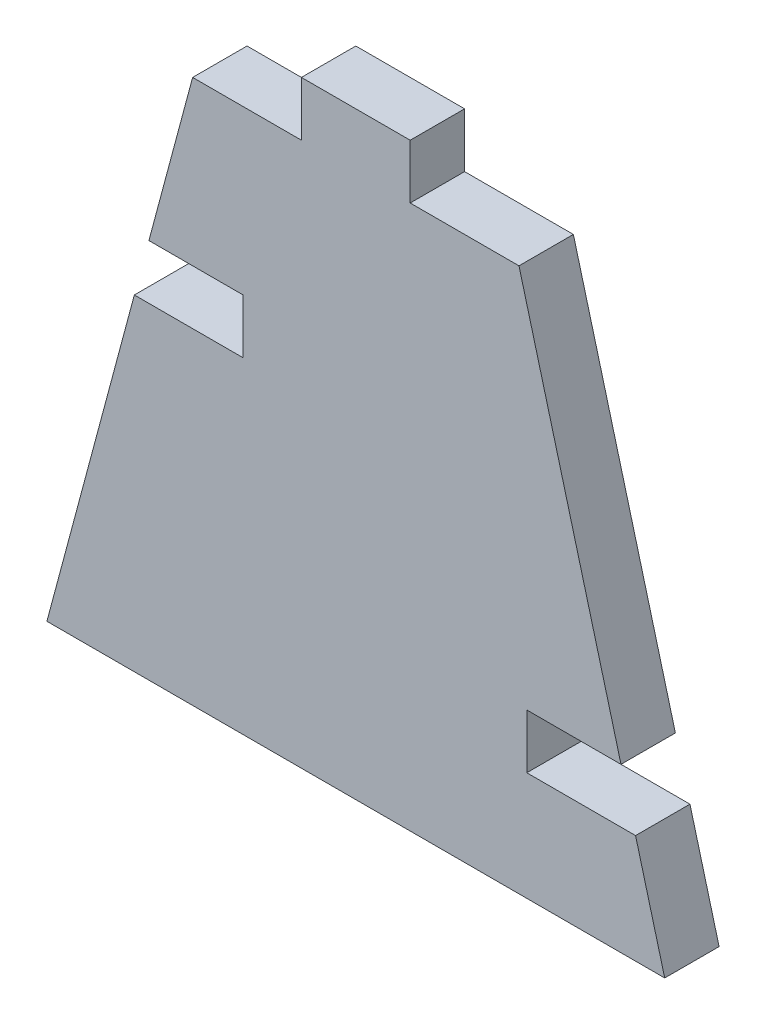
from build123d import *

# Parameters (mm, degrees)
LEG_PLATE_10MM_DEPTH = 5


with BuildPart() as part:
    # Leg Profile Sketch → Leg Plate 10mm (new, symmetric)
    with BuildSketch(Plane.XY):
        Polygon((0, 0), (113.589838486, 0), (108.230854638, 20), (88.230854638, 20), (88.230854638, 30), (105.551362713, 30), (86.794919243, 100), (66.794919243, 100), (66.794919243, 110), (46.794919243, 110), (46.794919243, 100), (26.794919243, 100), (18.75644347, 70), (36.076951546, 70), (36.076951546, 60), (16.076951546, 60), align=None)
    extrude(amount=LEG_PLATE_10MM_DEPTH, both=True)


solid = part.part
